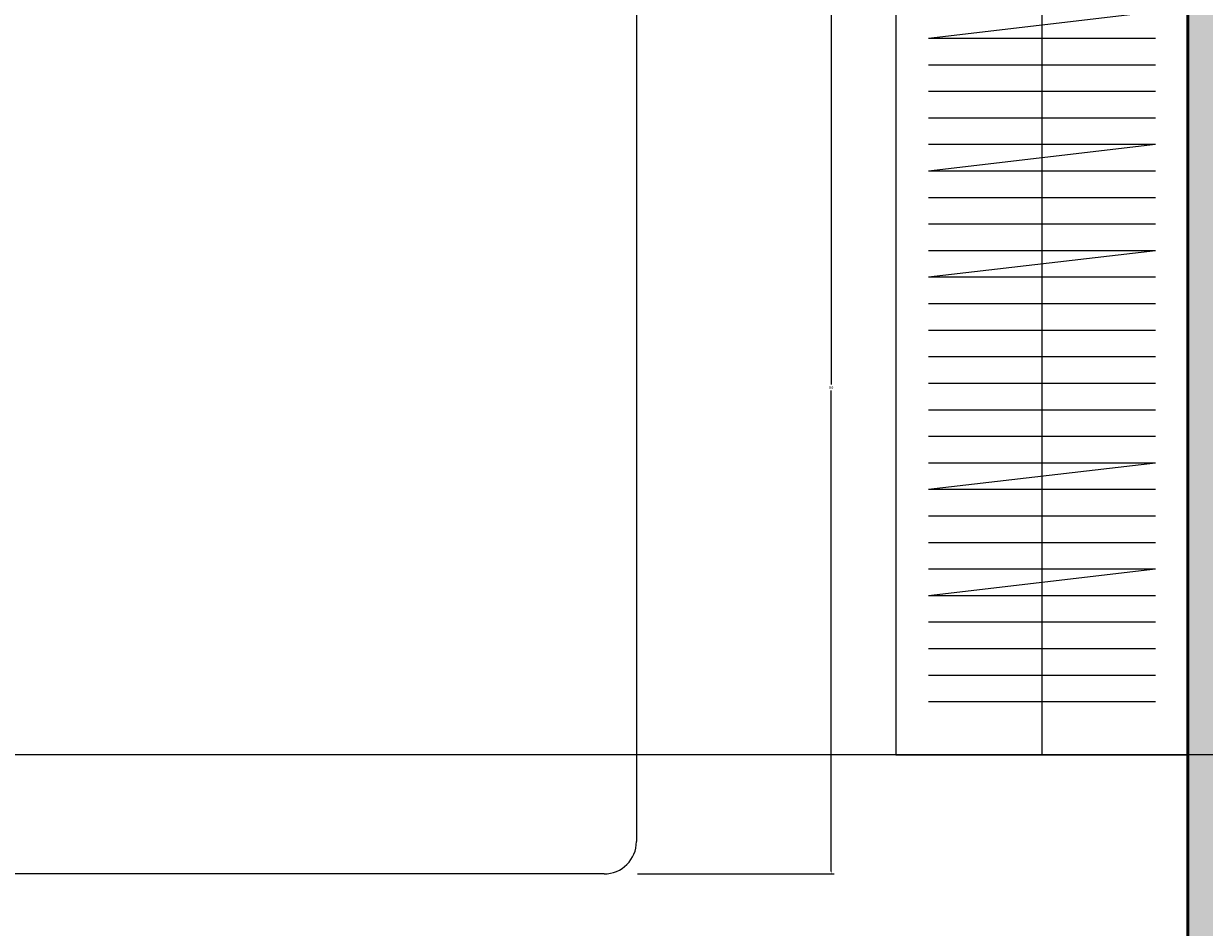
# Model space of a CAD drawing. Units: inches. Extents: x 2307 to 2544, y 2171 to 2540.
# Tile 25 of 52: x 2380 to 2453, y 2429 to 2485. Entities that reach past the tile are written whole.
import ezdxf

# ---------------------------------------------------------------- set-up
doc = ezdxf.new("R2010")
doc.units = ezdxf.units.IN
for name, color, linetype, lineweight in [('A-ANNO-DIMS', 2, 'Continuous', 18), ('A-FLOR-CASE', 9, 'Continuous', 18), ('A-FURN', 8, 'Continuous', 18), ('A-WALL', 7, 'Continuous', 50)]:
    doc.layers.add(name, color=color, linetype=linetype, lineweight=lineweight)
doc.layers.add('A-WALL-PATT', color=18, linetype='Continuous', lineweight=13, true_color=0x000000)
doc.styles.get("Standard").update_dxf_attribs({"font": 'arial.ttf'})
doc.dimstyles.get("Standard").update_dxf_attribs({"dimtxt": 0.18, "dimasz": 0.18, "dimexe": 0.18, "dimexo": 0.0625, "dimgap": 0.09, "dimtad": 0, "dimtih": 1, "dimtoh": 1, "dimdec": 4, "dimzin": 0, "dimdsep": 46, "dimtxsty": 'Standard', "dimcen": 0.09, "dimadec": 0, "dimazin": 0, "dimtfac": 1, "dimtdec": 4, "dimtofl": 0, "dimtmove": 0, "dimatfit": 3, "dimfxl": 1, "dimtolj": 1, "dimtzin": 0, "dimarcsym": 0})

# ---------------------------------------------------------------- blocks, each defined once
blk = doc.blocks.new('Bed - Queen')
for p, q in [((0, -78.00003), (0, -2)), ((57.99999, -80.00003), (2, -80.00003))]:
    blk.add_line(p, q)
blk.add_arc((2, -78.00003), 2, 180, 270)
blk = doc.blocks.new('WARDROBE-72X18IN')
for p, q in [((0, 72), (0, 0)), ((18, 72), (0, 72)), ((9, 72), (9, 0)), ((18, 0), (18, 72)), ((16, 68.727), (2, 68.727)), ((16, 68.727), (2, 67.09)), ((16, 67.09), (2, 67.09)), ((16, 65.454), (2, 65.454)), ((16, 63.818), (2, 63.818)), ((16, 62.181), (2, 62.181)), ((16, 62.181), (2, 60.545)), ((16, 60.545), (2, 60.545)), ((16, 58.909), (2, 58.909)), ((16, 57.272), (2, 57.272)), ((16, 57.272), (2, 55.636)), ((16, 55.636), (2, 55.636)), ((16, 54), (2, 54)), ((16, 52.363), (2, 52.363)), ((16, 50.727), (2, 50.727)), ((16, 49.09), (2, 49.09)), ((16, 47.454), (2, 47.454)), ((16, 45.818), (2, 45.818)), ((16, 45.818), (2, 44.181)), ((16, 44.181), (2, 44.181)), ((16, 42.545), (2, 42.545)), ((16, 40.909), (2, 40.909)), ((16, 39.272), (2, 39.272)), ((16, 37.636), (2, 37.636)), ((16, 37.636), (2, 36)), ((16, 36), (2, 36)), ((16, 34.363), (2, 34.363)), ((16, 32.727), (2, 32.727)), ((16, 31.09), (2, 31.09)), ((16, 31.09), (2, 29.454)), ((16, 29.454), (2, 29.454)), ((16, 27.818), (2, 27.818)), ((16, 26.181), (2, 26.181)), ((16, 24.545), (2, 24.545)), ((16, 22.909), (2, 22.909)), ((16, 21.272), (2, 21.272)), ((16, 19.636), (2, 19.636)), ((16, 18), (2, 18)), ((16, 18), (2, 16.363)), ((16, 16.363), (2, 16.363)), ((16, 14.727), (2, 14.727)), ((16, 13.09), (2, 13.09)), ((16, 11.454), (2, 11.454)), ((16, 11.454), (2, 9.818)), ((16, 9.818), (2, 9.818)), ((16, 8.181), (2, 8.181)), ((16, 6.545), (2, 6.545)), ((16, 4.909), (2, 4.909)), ((16, 3.272), (2, 3.272)), ((0, 0), (18, 0)), ((18, 0), (0, 0))]:
    blk.add_line(p, q)
blk = doc.blocks.new('*D27')
at = {"layer": 'A-ANNO-DIMS', "color": 0, "lineweight": -2, "transparency": 16777216}
for p, q in [((2417.771, 2492.174), (2429.888, 2492.174)), ((2429.708, 2491.994), (2429.708, 2462.356)), ((2429.708, 2432.354), (2429.708, 2461.992)), ((2417.771, 2432.174), (2429.888, 2432.174))]:
    blk.add_line(p, q, dxfattribs=at)
at = {"layer": 'A-ANNO-DIMS', "color": 0, "transparency": 16777216}
for points in [[(2429.678, 2491.994), (2429.738, 2491.994), (2429.708, 2492.174)], [(2429.678, 2432.354), (2429.738, 2432.354), (2429.708, 2432.174)]]:
    blk.add_solid(points, dxfattribs=at)
at = {"layer": 'Defpoints', "color": 0, "transparency": 16777216}
for p in [(2417.708, 2492.174), (2429.708, 2492.174), (2417.708, 2432.174)]:
    blk.add_point(p, dxfattribs=at)
at = {"layer": 'A-ANNO-DIMS', "color": 0, "transparency": 16777216, "insert": (2429.708, 2462.174), "char_height": 0.18, "attachment_point": 5}
blk.add_mtext('\\A1;60', dxfattribs=at)
blk = doc.blocks.new('*D48')
at = {"layer": 'A-ANNO-DIMS', "color": 0, "lineweight": -2, "transparency": 16777216}
for p, q in [((2455.633, 2511.51), (2307.366, 2511.51)), ((2307.546, 2511.33), (2307.546, 2475.69)), ((2307.546, 2439.69), (2307.546, 2475.329)), ((2455.633, 2439.51), (2307.366, 2439.51))]:
    blk.add_line(p, q, dxfattribs=at)
at = {"layer": 'A-ANNO-DIMS', "color": 0, "transparency": 16777216}
for points in [[(2307.516, 2511.33), (2307.576, 2511.33), (2307.546, 2511.51)], [(2307.516, 2439.69), (2307.576, 2439.69), (2307.546, 2439.51)]]:
    blk.add_solid(points, dxfattribs=at)
at = {"layer": 'Defpoints', "color": 0, "transparency": 16777216}
for p in [(2307.546, 2511.51), (2455.696, 2511.51), (2455.696, 2439.51)]:
    blk.add_point(p, dxfattribs=at)
at = {"layer": 'A-ANNO-DIMS', "color": 0, "transparency": 16777216, "insert": (2307.546, 2475.51), "char_height": 0.18, "attachment_point": 5}
blk.add_mtext('\\A1;72', dxfattribs=at)

msp = doc.modelspace()

# ---------------------------------------------------------------- hatches: boundary and pattern name
at = {"layer": 'A-WALL-PATT'}
h = msp.add_hatch(color=256, dxfattribs=at)
h.dxf.hatch_style = 1
h.paths.add_polyline_path([(2433.6935, 2199.5096), (2415.6423, 2199.5096), (2415.6423, 2190.5096), (2433.7832, 2190.5096)], flags=17)
h.paths.add_polyline_path([(2367.6423, 2199.5096), (2335.6958, 2199.5096), (2335.6958, 2307.3983), (2326.6958, 2307.3983), (2326.6958, 2190.5096), (2367.6423, 2190.5096)])
h.paths.add_polyline_path([(2524.6958, 2520.5096), (2496.7832, 2520.5096), (2496.7832, 2515.5149), (2472.7832, 2515.5149), (2472.7832, 2520.5096), (2415.4028, 2520.5096), (2415.4028, 2511.5096), (2451.6958, 2511.5096), (2451.6958, 2439.5096), (2451.6958, 2391.5096), (2445.6958, 2391.5096), (2445.6958, 2387.5096), (2455.6958, 2387.5096), (2455.6958, 2435.5096), (2461.6958, 2435.5096), (2461.6958, 2439.5096), (2455.6958, 2439.5096), (2455.6958, 2511.5096), (2515.6958, 2511.5096), (2515.6958, 2439.5096), (2491.6958, 2439.5096), (2491.6958, 2435.5096), (2515.6958, 2435.5096), (2515.6958, 2319.5096), (2451.6958, 2319.5096), (2451.6958, 2281.5096), (2481.6958, 2281.5096), (2481.6958, 2225.5096), (2485.6958, 2225.5096), (2485.6958, 2285.5096), (2455.6958, 2285.5096), (2455.6958, 2315.5096), (2515.6958, 2315.5096), (2515.6958, 2199.5096), (2469.6952, 2199.5096), (2469.785, 2190.5096), (2524.6958, 2190.5096)])

# ---------------------------------------------------------------- linework, layer by layer
at = {"layer": 'A-WALL'}
for p, q in [((2451.6958, 2391.5096), (2451.6958, 2511.5096)), ((2451.6958, 2435.5096), (2451.6958, 2391.5096))]:
    msp.add_line(p, q, dxfattribs=at)

# ---------------------------------------------------------------- block references
at = {"layer": 'A-FLOR-CASE'}
msp.add_blockref('WARDROBE-72X18IN', (2433.696, 2439.51), dxfattribs=at)
at = {"layer": 'A-FURN', "rotation": 90}
msp.add_blockref('Bed - Queen', (2337.7083, 2432.1742), dxfattribs=at)

# ---------------------------------------------------------------- dimensions: what is measured, and where the dimension line sits
at = {"layer": 'A-ANNO-DIMS'}
for base, p1, p2, picture, middle in [((2307.5458, 2511.5096), (2455.6958, 2439.5096), (2455.6958, 2511.5096), '*D48', (2307.5458, 2475.5096)), ((2429.7084, 2492.1742), (2417.7084, 2432.1742), (2417.7084, 2492.1742), '*D27', (2429.7084, 2462.1742))]:
    dim = msp.add_linear_dim(base=base, p1=p1, p2=p2, angle=90, dimstyle='Standard', override={"dimdec": 0, "dimlfac": 1, "dimrnd": 0, "dimzin": 0, "dimdsep": 46, "dimlunit": 2}, dxfattribs=at)
    dim.commit()
    dim.dimension.update_dxf_attribs({"geometry": picture, "text_midpoint": middle})

doc.saveas('drawing.dxf')
